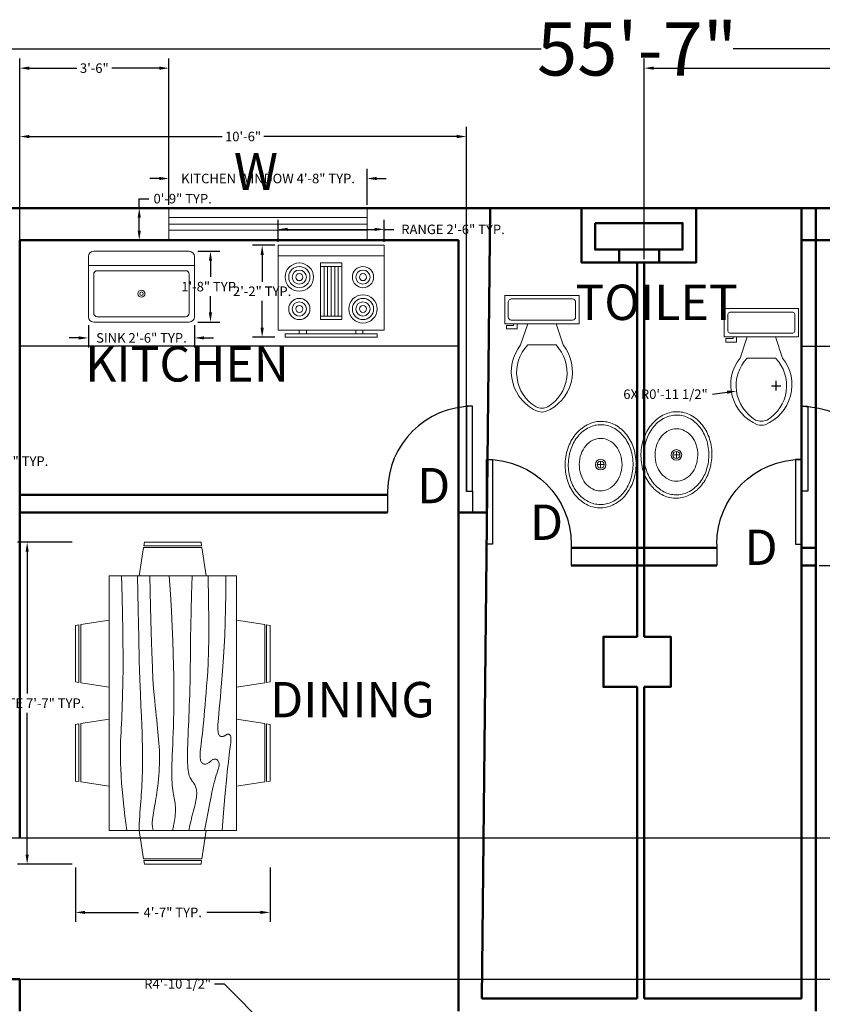
# Model space of a CAD drawing. Units: inches. Extents: x -15 to 796, y 111 to 651.
# Tile 4 of 6: x 189 to 416, y 373 to 651. Entities that reach past the tile are written whole.
import ezdxf

# ---------------------------------------------------------------- set-up
doc = ezdxf.new("R2010")
doc.units = ezdxf.units.IN
doc.header["$MEASUREMENT"] = 0
doc.layers.get('0').update_dxf_attribs({"color": 1})
for name, color, linetype, lineweight in [('A-ANNO-DIMS', 2, 'Continuous', 18), ('A-ANNO-TEXT', 7, 'Continuous', 18), ('A-AREA-IDEN', 7, 'Continuous', 25), ('A-COLS', 1, 'Continuous', 50), ('A-DOOR', 3, 'Continuous', 25), ('A-EQPM', 8, 'Continuous', 20), ('A-FLOR-CASE', 8, 'Continuous', 25), ('A-FLOR-FIXT', 9, 'Continuous', 20), ('A-FLOR-PATT', 18, 'Continuous', 13), ('A-FURN', 8, 'Continuous', 18), ('A-GLAZ', 4, 'Continuous', 18), ('A-WALL', 7, 'Continuous', 50)]:
    doc.layers.add(name, color=color, linetype=linetype, lineweight=lineweight)
doc.styles.get("Standard").update_dxf_attribs({"font": 'arial.ttf'})
doc.dimstyles.get("Standard").update_dxf_attribs({"dimscale": 15, "dimtxt": 0.18, "dimasz": 0.18, "dimexe": 0.18, "dimexo": 0.0625, "dimgap": 0.09, "dimtad": 0, "dimtih": 1, "dimtoh": 1, "dimdec": 0, "dimzin": 0, "dimdsep": 46, "dimlunit": 3, "dimtxsty": 'Standard', "dimcen": 0.09, "dimadec": 0, "dimazin": 0, "dimtfac": 1, "dimtdec": 0, "dimtofl": 0, "dimtmove": 0, "dimatfit": 3, "dimfxl": 1, "dimtolj": 1, "dimtzin": 0, "dimarcsym": 0})

# ---------------------------------------------------------------- blocks, each defined once
blk = doc.blocks.new('*U4')
for p, q in [((0, 0), (0, -6)), ((-40, 0), (-40, -6))]:
    blk.add_line(p, q)
blk.add_lwpolyline([(0, 0), (0, 40), (-1.75, 40), (-1.75, 0)], close=True)
blk.add_arc((0, 0), 40, 90, 180)
blk = doc.blocks.new('Range-Oven - 30 in top')
for p, q in [((0, -3), (30, -3)), ((12, -6), (18, -6)), ((13, -20), (13, -6)), ((14, -6), (14, -20)), ((15, -20), (15, -6)), ((16, -6), (16, -20)), ((17, -20), (17, -6)), ((18, -20), (12, -20)), ((6, -24), (6, -25)), ((8, -25), (8, -24)), ((22, -25), (22, -24)), ((24, -24), (24, -25))]:
    blk.add_line(p, q)
for points in [[(0, -24), (0, 0), (30, 0), (30, -24)], [(12, -21), (12, -5), (18, -5), (18, -21)], [(2, -26), (2, -25), (28, -25), (28, -26)]]:
    blk.add_lwpolyline(points, close=True)
for centre, radius in [((6, -9), 4), ((6, -9), 3), ((6, -9), 2), ((6, -9), 1), ((24, -9), 3), ((24, -9), 2), ((24, -9), 1), ((6, -18), 3), ((6, -18), 2), ((24, -18), 4), ((24, -18), 3), ((24, -18), 2), ((6, -18), 1), ((24, -18), 1)]:
    blk.add_circle(centre, radius)
blk = doc.blocks.new('Sink-single - 30 in top')
blk.add_line((-15, -3.999996), (15, -3.999996))
for points in [[(-13.5, 0), (13.5, 0)], [(-15, -18.499996), (-15, -1.5)], [(15, -1.5), (15, -18.499996)], [(-12.5, -5.499996), (12.5, -5.499996)], [(-13.5, -17.499996), (-13.5, -6.499996)], [(13.5, -6.499996), (13.5, -17.499996)], [(12.5, -18.499996), (-12.5, -18.499996)], [(13.5, -19.999996), (-13.5, -19.999996)]]:
    blk.add_lwpolyline(points)
for radius in [1, 0.5]:
    blk.add_circle((0, -11.999996), radius)
for centre, radius, start, end in [((-13.5, -1.5), 1.5, 90, 180), ((13.5, -1.5), 1.5, 0, 90), ((-12.5, -6.499996), 1, 90, 180), ((12.5, -6.499996), 1, 0, 90), ((-13.5, -18.499996), 1.5, 180, 270), ((-12.5, -17.499996), 1, 180, 270), ((12.5, -17.499996), 1, 270, 0), ((13.5, -18.499996), 1.5, 270, 0)]:
    blk.add_arc(centre, radius, start, end)
blk = doc.blocks.new('*U13')
for p, q in [((-24, 0), (-24, -6)), ((0, 0), (0, -6))]:
    blk.add_line(p, q)
blk.add_lwpolyline([(0, 0), (0, 24), (-1.75, 24), (-1.75, 0)], close=True)
blk.add_arc((0, 0), 24, 90, 180)
blk = doc.blocks.new('Dining Set - 36 x 72 in.')
for p, q in [((-22.2343, 26.00059), (-23.4847, 17.99762)), ((-22.2304, 26), (-5.7608, 26)), ((-22, 27.5), (-22.1562, 26.50042)), ((-5.8416, 26.5), (-22.1534, 26.5)), ((-22, 27.5), (-6, 27.5)), ((-5.8437, 26.49966), (-6, 27.5)), ((-4.5152, 17.99762), (-5.7655, 25.99926)), ((5.7657, 26.00059), (4.5153, 17.99762)), ((5.7696, 26), (22.2392, 26)), ((6, 27.5), (5.8438, 26.50042)), ((22.1584, 26.5), (5.8466, 26.5)), ((6, 27.5), (22, 27.5)), ((22.1563, 26.49966), (22, 27.5)), ((23.4848, 17.99762), (22.2345, 25.99926)), ((36, 18), (-36, 18)), ((-36, 18), (-36, -18)), ((36, -18), (36, 18)), ((-44.0006, 8.23428), (-35.9976, 9.48474)), ((44.0006, 8.23428), (35.9976, 9.48474)), ((-45.5, 8), (-44.5004, 8.15617)), ((-45.5, 8), (-45.5, -8)), ((-44.5, -8.15843), (-44.5, 8.15338)), ((-44, 8.23041), (-44, -8.23915)), ((44, 8.23041), (44, -8.23915)), ((44.5, -8.15843), (44.5, 8.15338)), ((45.5, 8), (44.5005, 8.15617)), ((45.5, 8), (45.5, -8)), ((-44.4997, -8.15631), (-45.5, -8)), ((-35.9976, -9.48476), (-43.9993, -8.2345)), ((35.9976, -9.48476), (43.9993, -8.2345)), ((44.4997, -8.15631), (45.5, -8)), ((-36, -18), (36, -18)), ((-22.2343, -26.0006), (-23.4847, -17.99762)), ((-4.5152, -17.99762), (-5.7655, -25.99928)), ((5.7657, -26.0006), (4.5153, -17.99762)), ((23.4848, -17.99762), (22.2345, -25.99928)), ((-22.2304, -26), (-5.7608, -26)), ((-22, -27.5), (-22.1562, -26.50044)), ((-5.8416, -26.5), (-22.1534, -26.5)), ((-22, -27.5), (-6, -27.5)), ((-5.8437, -26.49967), (-6, -27.5)), ((5.7696, -26), (22.2392, -26)), ((6, -27.5), (5.8438, -26.50044)), ((22.1584, -26.5), (5.8466, -26.5)), ((6, -27.5), (22, -27.5)), ((22.1563, -26.49967), (22, -27.5))]:
    blk.add_line(p, q)
for points in [[(-36, 15), (-31.1772, 14.97754), (-26.8079, 14.91406), (-22.8538, 14.81543), (-19.276, 14.6875), (-16.0362, 14.53613), (-13.0957, 14.36718), (-10.4159, 14.18652), (-7.9583, 14), (-5.6904, 13.81315), (-3.6035, 13.63021), (-1.6954, 13.45508), (0.0365, 13.29166), (1.5945, 13.14388), (2.9811, 13.01562), (4.1988, 12.9108), (5.25, 12.83333), (6.1393, 12.78613), (6.8802, 12.76823), (7.4883, 12.77767), (7.9792, 12.8125), (8.3685, 12.87077), (8.6719, 12.95052), (8.9049, 13.0498), (9.0833, 13.16666), (9.2205, 13.29899), (9.3216, 13.44401), (9.3895, 13.59879), (9.4271, 13.76041), (9.4373, 13.92594), (9.4232, 14.09245), (9.3875, 14.257), (9.3333, 14.41666), (9.2638, 14.56917), (9.1836, 14.71484), (9.0975, 14.85465), (9.0104, 14.98958), (8.9272, 15.1206), (8.8529, 15.2487), (8.7922, 15.37483), (8.75, 15.5), (8.7305, 15.62467), (8.7344, 15.74739), (8.7617, 15.86621), (8.8125, 15.97916), (8.8867, 16.08431), (8.9844, 16.17968), (9.1055, 16.26334), (9.25, 16.33333), (9.4189, 16.38802), (9.6172, 16.42708), (9.8506, 16.45052), (10.125, 16.45833), (10.4463, 16.45052), (10.8203, 16.42708), (11.2529, 16.38802), (11.75, 16.33333), (12.3184, 16.26318), (12.9694, 16.17838), (13.7151, 16.07991), (14.5677, 15.96875), (15.5395, 15.84586), (16.6426, 15.71224), (17.8893, 15.56884), (19.2917, 15.41666), (20.859, 15.25667), (22.5879, 15.08984), (24.4721, 14.91715), (26.5052, 14.73958), (28.6809, 14.5581), (30.9929, 14.3737), (33.4347, 14.18733), (36, 14)], [(-36, 10), (-28.9766, 10.14274), (-23.1725, 10.20442), (-18.4241, 10.19775), (-14.5677, 10.13541), (-11.4399, 10.03011), (-8.877, 9.89453), (-6.7154, 9.74137), (-4.7917, 9.58333), (-2.9698, 9.43082), (-1.2246, 9.28515), (0.4415, 9.14534), (2.026, 9.01041), (3.5266, 8.87939), (4.9408, 8.7513), (6.266, 8.62516), (7.5, 8.5), (8.6411, 8.37549), (9.6914, 8.2539), (10.6538, 8.13818), (11.5312, 8.03125), (12.3267, 7.93603), (13.043, 7.85547), (13.6831, 7.79248), (14.25, 7.75), (14.7471, 7.7303), (15.1797, 7.73307), (15.5537, 7.75732), (15.875, 7.80208), (16.1494, 7.86637), (16.3828, 7.94922), (16.5811, 8.04964), (16.75, 8.16666), (16.8944, 8.29915), (17.0143, 8.44531), (17.1089, 8.60319), (17.1771, 8.77083), (17.218, 8.94629), (17.2305, 9.1276), (17.2137, 9.31282), (17.1667, 9.5), (17.0895, 9.6875), (16.987, 9.875), (16.8649, 10.0625), (16.7292, 10.25), (16.5856, 10.4375), (16.4401, 10.625), (16.2985, 10.8125), (16.1667, 11), (16.05, 11.18733), (15.9518, 11.3737), (15.8752, 11.5581), (15.8229, 11.73958), (15.798, 11.91715), (15.8034, 12.08984), (15.842, 12.25667), (15.9167, 12.41666), (16.0295, 12.56836), (16.1784, 12.70833), (16.3605, 12.83268), (16.5729, 12.9375), (16.8127, 13.01888), (17.0768, 13.07291), (17.3625, 13.0957), (17.6667, 13.08333), (17.9894, 13.03312), (18.3418, 12.94726), (18.7382, 12.82918), (19.1927, 12.68229), (19.7195, 12.51001), (20.3327, 12.31575), (21.0465, 12.10294), (21.875, 11.875), (22.8357, 11.63354), (23.959, 11.37304), (25.2786, 11.08618), (26.8282, 10.76562), (28.6414, 10.40405), (30.752, 9.99414), (33.1936, 9.52856), (36, 9)], [(-36, 5.5), (-30.7157, 5.3348), (-26.069, 5.20963), (-21.9946, 5.11767), (-18.4271, 5.05208), (-15.3009, 5.00602), (-12.5508, 4.97265), (-10.1112, 4.94515), (-7.9167, 4.91666), (-5.909, 4.88167), (-4.0586, 4.83984), (-2.3429, 4.79215), (-0.7396, 4.73958), (0.7739, 4.6831), (2.22, 4.6237), (3.6213, 4.56233), (5, 4.5), (6.373, 4.43782), (7.7344, 4.3776), (9.0723, 4.32129), (10.375, 4.27083), (11.6309, 4.22819), (12.8281, 4.19531), (13.9551, 4.17415), (15, 4.16666), (15.954, 4.17448), (16.819, 4.19791), (17.6001, 4.23698), (18.3021, 4.29166), (18.9299, 4.36198), (19.4883, 4.44791), (19.9823, 4.54948), (20.4167, 4.66666), (20.7969, 4.79899), (21.1302, 4.94401), (21.4245, 5.09879), (21.6875, 5.26041), (21.9271, 5.42594), (22.1511, 5.59245), (22.3672, 5.757), (22.5834, 5.91666), (22.8065, 6.06868), (23.0404, 6.21093), (23.2879, 6.34147), (23.5521, 6.45833), (23.8358, 6.55957), (24.142, 6.64323), (24.4735, 6.70735), (24.8334, 6.75), (25.2235, 6.76969), (25.642, 6.76692), (26.0858, 6.74267), (26.5521, 6.69791), (27.0379, 6.63362), (27.5404, 6.55078), (28.0565, 6.45036), (28.5834, 6.33333), (29.1242, 6.19987), (29.7071, 6.04687), (30.3661, 5.87044), (31.1354, 5.66666), (32.0493, 5.43164), (33.142, 5.16146), (34.4475, 4.85221), (36, 4.5)], [(-36, -1), (-30.7915, -0.6591), (-26.0195, -0.38216), (-21.6519, -0.16284), (-17.6563, 0.00521), (-14.0005, 0.12833), (-10.6523, 0.21289), (-7.5796, 0.26522), (-4.75, 0.29166), (-2.134, 0.29793), (0.2878, 0.28711), (2.5317, 0.26163), (4.6146, 0.22396), (6.5529, 0.17651), (8.3633, 0.12174), (10.0623, 0.06209), (11.6667, 0), (13.1899, -0.06201), (14.6341, -0.1211), (15.9982, -0.17432), (17.2813, -0.21875), (18.4823, -0.25147), (19.6003, -0.26953), (20.6343, -0.27002), (21.5834, -0.25), (22.4481, -0.20768), (23.2357, -0.14584), (23.9549, -0.06836), (24.6146, 0.02083), (25.2235, 0.11784), (25.7904, 0.21875), (26.3241, 0.31966), (26.8334, 0.41666), (27.3265, 0.50618), (27.8099, 0.58593), (28.2894, 0.65397), (28.7709, 0.70833), (29.2601, 0.74707), (29.763, 0.76823), (30.2855, 0.76985), (30.8334, 0.75), (31.4088, 0.70784), (31.9994, 0.64713), (32.589, 0.57275), (33.1615, 0.48958), (33.7008, 0.4025), (34.1908, 0.3164), (34.6153, 0.23616), (34.9584, 0.16666), (35.2099, 0.11165), (35.3848, 0.07031), (35.504, 0.04069), (35.5886, 0.02083), (35.6594, 0.00879), (35.7377, 0.0026), (35.8442, 0.00032), (36, 0)], [(-36, -6.5), (-27.1843, -6.31267), (-20.084, -6.1263), (-14.469, -5.9419), (-10.1094, -5.76042), (-6.7752, -5.58285), (-4.2363, -5.41016), (-2.2629, -5.24333), (-0.625, -5.08334), (0.8708, -4.93099), (2.2715, -4.78646), (3.5872, -4.64974), (4.8281, -4.52084), (6.0046, -4.39974), (7.127, -4.28646), (8.2053, -4.18099), (9.25, -4.08334), (10.2705, -3.99382), (11.2734, -3.91407), (12.2647, -3.84603), (13.25, -3.79167), (14.2354, -3.75293), (15.2266, -3.73177), (16.2295, -3.73015), (17.25, -3.75), (18.2912, -3.79248), (19.3451, -3.85547), (20.4009, -3.93604), (21.4479, -4.03125), (22.4754, -4.13819), (23.4727, -4.25391), (24.4289, -4.37549), (25.3334, -4.5), (26.1785, -4.62492), (26.9694, -4.74935), (27.7145, -4.87281), (28.4219, -4.99479), (29.1, -5.11483), (29.7572, -5.23242), (30.4016, -5.34709), (31.0417, -5.45834), (31.6837, -5.56437), (32.3262, -5.65821), (32.9658, -5.73153), (33.599, -5.77604), (34.2224, -5.78345), (34.8327, -5.74545), (35.4264, -5.65373), (36, -5.5)], [(-36, -10), (-26.4022, -9.81299), (-18.4675, -9.62891), (-11.9839, -9.45069), (-6.7396, -9.28125), (-2.5226, -9.12354), (0.8789, -8.98047), (3.6769, -8.85498), (6.0833, -8.75), (8.2767, -8.66765), (10.3021, -8.60677), (12.1712, -8.56543), (13.8958, -8.54167), (15.4876, -8.53353), (16.9583, -8.53907), (18.3197, -8.55632), (19.5834, -8.58334), (20.7616, -8.61841), (21.8685, -8.66081), (22.9188, -8.71004), (23.9271, -8.76563), (24.9081, -8.82707), (25.8763, -8.89388), (26.8465, -8.96558), (27.8334, -9.04167), (28.8474, -9.12118), (29.8828, -9.20117), (30.93, -9.27824), (31.9792, -9.34896), (33.0205, -9.40991), (34.0443, -9.45768), (35.0407, -9.48885), (36, -9.5)], [(-36, -14.5), (-30.0881, -14.33513), (-25.0332, -14.21224), (-20.7312, -14.12647), (-17.0781, -14.07292), (-13.97, -14.04671), (-11.3027, -14.04297), (-8.9724, -14.05681), (-6.875, -14.08334), (-4.9224, -14.11833), (-3.0905, -14.16016), (-1.3709, -14.20785), (0.2448, -14.26042), (1.7647, -14.3169), (3.1973, -14.3763), (4.5507, -14.43767), (5.8333, -14.5), (7.0554, -14.5621), (8.235, -14.62175), (9.3922, -14.67652), (10.5469, -14.72396), (11.7192, -14.76164), (12.929, -14.78711), (14.1965, -14.79794), (15.5417, -14.79167), (16.9933, -14.76424), (18.6152, -14.70508), (20.4804, -14.60197), (22.6615, -14.44271), (25.2312, -14.21509), (28.2624, -13.9069), (31.8277, -13.50594), (36, -13)]]:
    blk.add_lwpolyline(points)
blk = doc.blocks.new('Sink - Oval top')
for p, q in [((-1, 0), (1, 0)), ((0, 1), (0, -1))]:
    blk.add_line(p, q)
for points in [[(-12.23, 0.39, 0.117634), (-11.46, -3.36, 0.104469), (-8.88, -6.8, 0.090016), (-5.08, -9.07, 0.08192), (-0.32, -10.02, 0.08192), (4.49, -9.38, 0.090016), (8.42, -7.36, 0.104469), (11.22, -4.09, 0.117634), (12.23, -0.39, 0.117634), (11.46, 3.36, 0.104469), (8.88, 6.8, 0.090016), (5.08, 9.07, 0.08192), (0.32, 10.02, 0.08192), (-4.49, 9.38, 0.090016), (-8.42, 7.36, 0.104469), (-11.22, 4.09, 0.117634)], [(-11.29, 0.16, 0.118622), (-10.52, -3.25, 0.104678), (-8.07, -6.36, 0.089562), (-4.54, -8.37, 0.081185), (-0.13, -9.15, 0.081185), (4.3, -8.49, 0.089562), (7.89, -6.58, 0.104678), (10.42, -3.55, 0.118622), (11.29, -0.16, 0.118622), (10.52, 3.25, 0.104678), (8.07, 6.36, 0.089562), (4.54, 8.37, 0.081185), (0.13, 9.15, 0.081185), (-4.3, 8.49, 0.089562), (-7.89, 6.58, 0.104678), (-10.42, 3.55, 0.118622)], [(-7.42, 0.08, 0.118283), (-6.91, -2.17, 0.104607), (-5.29, -4.21, 0.089718), (-2.97, -5.53, 0.081436), (-0.07, -6.04, 0.081436), (2.84, -5.59, 0.089718), (5.2, -4.33, 0.104607), (6.86, -2.32, 0.118283), (7.42, -0.08, 0.118283), (6.91, 2.17, 0.104607), (5.29, 4.21, 0.089718), (2.97, 5.53, 0.081436), (0.07, 6.04, 0.081436), (-2.84, 5.59, 0.089718), (-5.2, 4.33, 0.104607), (-6.86, 2.32, 0.118283)]]:
    blk.add_lwpolyline(points, format="xyb", close=True)
for radius in [1.5, 1]:
    blk.add_circle((0, 0), radius)
blk = doc.blocks.new('Toilet - top')
for p, q in [((9.5, -6), (9.5, -2)), ((-8, -8.5), (-8, -8)), ((-7, -8), (-7, -9.5)), ((-4, -8), (-6, -14)), ((4, -8), (6, -14)), ((-10, -8.5), (-8, -8.5)), ((-10, -9.5), (-10, -8.5)), ((-7, -9.5), (-10, -9.5)), ((4, -14), (-4, -14))]:
    blk.add_line(p, q)
blk.add_lwpolyline([(10.5, -8), (10.5, 0), (-10.5, 0), (-10.5, -8)], close=True)
for points in [[(-9.5, -2), (-9.5, -6)], [(8.5, -1), (-8.5, -1)], [(-8.5, -7), (8.5, -7)]]:
    blk.add_lwpolyline(points)
for centre, radius, start, end in [((-8.62, -1.88), 0.884, 81.8699, 188.1301), ((8.62, -1.88), 0.884, 351.8699, 98.1301), ((-8.62, -6.12), 0.884, 171.8699, 278.1301), ((8.62, -6.12), 0.884, 261.8699, 8.1301), ((3.52, -21.58), 12.17, 141.4691, 247.9714), ((4.2, -21.82), 11.33, 136.3677, 238.9468), ((-3.52, -21.58), 12.17, 292.0284, 38.5307), ((-4.2, -21.82), 11.33, 301.053, 43.6321), ((0, -27.88), 4, 245.7318, 294.2682), ((0, -29), 4, 254.8605, 285.1395)]:
    blk.add_arc(centre, radius, start, end)
blk = doc.blocks.new('*U15')
for p, q in [((0, 0), (0, -6)), ((24, 0), (24, -6))]:
    blk.add_line(p, q)
blk.add_lwpolyline([(0, 0), (0, 24), (1.75, 24), (1.75, 0)], close=True)
blk.add_arc((0, 0), 24, 0, 90)
blk = doc.blocks.new('*D16')
at = {"layer": 'A-ANNO-DIMS', "color": 0, "lineweight": -2, "transparency": 16777216}
for p, q in [((30.18, 599.06), (30.18, 645.85)), ((697.18, 599.06), (697.18, 645.85)), ((32.88, 643.15), (336.57, 643.15)), ((694.48, 643.15), (390.8, 643.15))]:
    blk.add_line(p, q, dxfattribs=at)
at = {"layer": 'A-ANNO-DIMS', "color": 0, "transparency": 16777216}
for points in [[(32.88, 643.6), (32.88, 642.7), (30.18, 643.15)], [(694.48, 643.6), (694.48, 642.7), (697.18, 643.15)]]:
    blk.add_solid(points, dxfattribs=at)
at = {"layer": 'Defpoints', "color": 0, "transparency": 16777216}
for p in [(697.18, 643.15), (30.18, 598.13), (697.18, 598.13)]:
    blk.add_point(p, dxfattribs=at)
at = {"layer": 'A-ANNO-DIMS', "color": 0, "transparency": 16777216, "insert": (363.68, 643.15), "char_height": 2.7, "attachment_point": 5}
blk.add_mtext('\\A1;{\\H5.55556x;55\'-7"}', dxfattribs=at)
blk = doc.blocks.new('*D22')
at = {"layer": 'A-ANNO-DIMS', "color": 0, "lineweight": -2, "transparency": 16777216}
for p, q in [((189.18, 518.06), (189.18, 621.1)), ((315.43, 518.06), (315.43, 621.1)), ((191.88, 618.4), (246.45, 618.4)), ((312.73, 618.4), (258.17, 618.4))]:
    blk.add_line(p, q, dxfattribs=at)
at = {"layer": 'A-ANNO-DIMS', "color": 0, "transparency": 16777216}
for points in [[(191.88, 618.85), (191.88, 617.95), (189.18, 618.4)], [(312.73, 618.85), (312.73, 617.95), (315.43, 618.4)]]:
    blk.add_solid(points, dxfattribs=at)
at = {"layer": 'Defpoints', "color": 0, "transparency": 16777216}
for p in [(315.43, 618.4), (189.18, 517.13), (315.43, 517.13)]:
    blk.add_point(p, dxfattribs=at)
at = {"layer": 'A-ANNO-DIMS', "color": 0, "transparency": 16777216, "insert": (252.31, 618.4), "char_height": 2.7, "attachment_point": 5}
blk.add_mtext('\\A1;10\'-6"', dxfattribs=at)
blk = doc.blocks.new('WIN-KITCHEN-56IN')
for p, q in [((0, 6.34), (56, 6.34)), ((0, 4.5), (56, 4.5)), ((0, 2.84), (56, 2.84))]:
    blk.add_line(p, q)
blk.add_lwpolyline([(0, 9), (56, 9), (56, 0), (0, 0)], close=True)
blk = doc.blocks.new('*D45')
at = {"layer": 'A-ANNO-DIMS', "color": 0, "lineweight": -2, "transparency": 16777216}
for p, q in [((134.03, 529.37), (134.03, 523.92)), ((158.58, 529.37), (158.58, 523.92)), ((136.73, 526.62), (155.88, 526.62)), ((158.58, 526.62), (161.28, 526.62))]:
    blk.add_line(p, q, dxfattribs=at)
at = {"layer": 'A-ANNO-DIMS', "color": 0, "transparency": 16777216}
for points in [[(136.73, 527.07), (136.73, 526.17), (134.03, 526.62)], [(155.88, 527.07), (155.88, 526.17), (158.58, 526.62)]]:
    blk.add_solid(points, dxfattribs=at)
at = {"layer": 'Defpoints', "color": 0, "transparency": 16777216}
for p in [(134.03, 530.3), (158.58, 530.3), (158.58, 526.62)]:
    blk.add_point(p, dxfattribs=at)
at = {"layer": 'A-ANNO-DIMS', "color": 0, "transparency": 16777216, "insert": (180.13, 526.62), "char_height": 2.7, "attachment_point": 5}
blk.add_mtext('\\A1;BASIN 2\'-0 1/2" TYP.', dxfattribs=at)
blk = doc.blocks.new('*D51')
at = {"layer": 'A-ANNO-DIMS', "color": 0, "lineweight": -2, "transparency": 16777216}
for p, q in [((262.21, 588.59), (262.21, 594.85)), ((292.21, 588.59), (292.21, 594.85)), ((264.91, 592.15), (289.51, 592.15)), ((292.21, 592.15), (294.91, 592.15))]:
    blk.add_line(p, q, dxfattribs=at)
at = {"layer": 'A-ANNO-DIMS', "color": 0, "transparency": 16777216}
for points in [[(264.91, 592.6), (264.91, 591.7), (262.21, 592.15)], [(289.51, 592.6), (289.51, 591.7), (292.21, 592.15)]]:
    blk.add_solid(points, dxfattribs=at)
at = {"layer": 'Defpoints', "color": 0, "transparency": 16777216}
for p in [(292.21, 592.15), (262.21, 587.65), (292.21, 587.65)]:
    blk.add_point(p, dxfattribs=at)
at = {"layer": 'A-ANNO-DIMS', "color": 0, "transparency": 16777216, "insert": (311.65, 592.15), "char_height": 2.7, "attachment_point": 5}
blk.add_mtext('\\A1;RANGE 2\'-6" TYP.', dxfattribs=at)
blk = doc.blocks.new('*D52')
at = {"layer": 'A-ANNO-DIMS', "color": 0, "lineweight": -2, "transparency": 16777216}
for p, q in [((261.28, 587.65), (255.01, 587.65)), ((257.71, 584.95), (257.71, 577.36)), ((257.71, 564.35), (257.71, 571.94)), ((261.28, 561.65), (255.01, 561.65))]:
    blk.add_line(p, q, dxfattribs=at)
at = {"layer": 'A-ANNO-DIMS', "color": 0, "transparency": 16777216}
for points in [[(257.26, 584.95), (258.16, 584.95), (257.71, 587.65)], [(257.26, 564.35), (258.16, 564.35), (257.71, 561.65)]]:
    blk.add_solid(points, dxfattribs=at)
at = {"layer": 'Defpoints', "color": 0, "transparency": 16777216}
for p in [(257.71, 587.65), (262.21, 587.65), (262.21, 561.65)]:
    blk.add_point(p, dxfattribs=at)
at = {"layer": 'A-ANNO-DIMS', "color": 0, "transparency": 16777216, "insert": (257.71, 574.65), "char_height": 2.7, "attachment_point": 5}
blk.add_mtext('\\A1;2\'-2" TYP.', dxfattribs=at)
blk = doc.blocks.new('*D53')
at = {"layer": 'A-ANNO-DIMS', "color": 0, "lineweight": -2, "transparency": 16777216}
for p, q in [((208.59, 565.02), (208.59, 558.76)), ((238.59, 565.02), (238.59, 558.76)), ((205.89, 561.46), (203.19, 561.46)), ((241.29, 561.46), (243.99, 561.46))]:
    blk.add_line(p, q, dxfattribs=at)
at = {"layer": 'A-ANNO-DIMS', "color": 0, "transparency": 16777216}
for points in [[(205.89, 561.91), (205.89, 561.01), (208.59, 561.46)], [(241.29, 561.91), (241.29, 561.01), (238.59, 561.46)]]:
    blk.add_solid(points, dxfattribs=at)
at = {"layer": 'Defpoints', "color": 0, "transparency": 16777216}
for p in [(208.59, 565.96), (238.59, 565.96), (238.59, 561.46)]:
    blk.add_point(p, dxfattribs=at)
at = {"layer": 'A-ANNO-DIMS', "color": 0, "transparency": 16777216, "insert": (223.59, 561.46), "char_height": 2.7, "attachment_point": 5}
blk.add_mtext('\\A1;SINK 2\'-6" TYP.', dxfattribs=at)
blk = doc.blocks.new('*D54')
at = {"layer": 'A-ANNO-DIMS', "color": 0, "lineweight": -2, "transparency": 16777216}
for p, q in [((239.53, 585.96), (245.79, 585.96)), ((243.09, 583.26), (243.09, 578.69)), ((243.09, 568.66), (243.09, 573.23)), ((239.53, 565.96), (245.79, 565.96))]:
    blk.add_line(p, q, dxfattribs=at)
at = {"layer": 'A-ANNO-DIMS', "color": 0, "transparency": 16777216}
for points in [[(242.64, 583.26), (243.54, 583.26), (243.09, 585.96)], [(242.64, 568.66), (243.54, 568.66), (243.09, 565.96)]]:
    blk.add_solid(points, dxfattribs=at)
at = {"layer": 'Defpoints', "color": 0, "transparency": 16777216}
for p in [(238.59, 585.96), (243.09, 585.96), (238.59, 565.96)]:
    blk.add_point(p, dxfattribs=at)
at = {"layer": 'A-ANNO-DIMS', "color": 0, "transparency": 16777216, "insert": (243.09, 575.96), "char_height": 2.7, "attachment_point": 5}
blk.add_mtext('\\A1;1\'-8" TYP.', dxfattribs=at)
blk = doc.blocks.new('*D55')
at = {"layer": 'A-ANNO-DIMS', "color": 0, "lineweight": -2, "transparency": 16777216}
for p, q in [((204, 503.69), (188.59, 503.69)), ((191.29, 500.99), (191.29, 460.89)), ((191.29, 415.39), (191.29, 455.48)), ((204, 412.69), (188.59, 412.69))]:
    blk.add_line(p, q, dxfattribs=at)
at = {"layer": 'A-ANNO-DIMS', "color": 0, "transparency": 16777216}
for points in [[(190.84, 500.99), (191.74, 500.99), (191.29, 503.69)], [(190.84, 415.39), (191.74, 415.39), (191.29, 412.69)]]:
    blk.add_solid(points, dxfattribs=at)
at = {"layer": 'Defpoints', "color": 0, "transparency": 16777216}
for p in [(204.94, 503.69), (191.29, 412.69), (204.94, 412.69)]:
    blk.add_point(p, dxfattribs=at)
at = {"layer": 'A-ANNO-DIMS', "color": 0, "transparency": 16777216, "insert": (191.29, 458.19), "char_height": 2.7, "attachment_point": 5}
blk.add_mtext('\\A1;DINETTE 7\'-7" TYP.', dxfattribs=at)
blk = doc.blocks.new('*D56')
at = {"layer": 'A-ANNO-DIMS', "color": 0, "lineweight": -2, "transparency": 16777216}
for p, q in [((204.94, 411.75), (204.94, 396.34)), ((259.94, 411.75), (259.94, 396.34)), ((207.64, 399.04), (222.8, 399.04)), ((257.24, 399.04), (242.07, 399.04))]:
    blk.add_line(p, q, dxfattribs=at)
at = {"layer": 'A-ANNO-DIMS', "color": 0, "transparency": 16777216}
for points in [[(207.64, 399.49), (207.64, 398.59), (204.94, 399.04)], [(257.24, 399.49), (257.24, 398.59), (259.94, 399.04)]]:
    blk.add_solid(points, dxfattribs=at)
at = {"layer": 'Defpoints', "color": 0, "transparency": 16777216}
for p in [(204.94, 412.69), (259.94, 412.69), (259.94, 399.04)]:
    blk.add_point(p, dxfattribs=at)
at = {"layer": 'A-ANNO-DIMS', "color": 0, "transparency": 16777216, "insert": (232.44, 399.04), "char_height": 2.7, "attachment_point": 5}
blk.add_mtext('\\A1;4\'-7" TYP.', dxfattribs=at)
blk = doc.blocks.new('*D61')
at = {"layer": 'A-ANNO-DIMS', "color": 0, "lineweight": -2, "transparency": 16777216}
for p, q in [((231.37, 599.06), (231.37, 609.23)), ((287.37, 599.06), (287.37, 609.23)), ((228.67, 606.53), (225.97, 606.53)), ((290.07, 606.53), (292.77, 606.53))]:
    blk.add_line(p, q, dxfattribs=at)
at = {"layer": 'A-ANNO-DIMS', "color": 0, "transparency": 16777216}
for points in [[(228.67, 606.98), (228.67, 606.08), (231.37, 606.53)], [(290.07, 606.98), (290.07, 606.08), (287.37, 606.53)]]:
    blk.add_solid(points, dxfattribs=at)
at = {"layer": 'Defpoints', "color": 0, "transparency": 16777216}
for p in [(287.37, 606.53), (231.37, 598.13), (287.37, 598.13)]:
    blk.add_point(p, dxfattribs=at)
at = {"layer": 'A-ANNO-DIMS', "color": 0, "transparency": 16777216, "insert": (259.37, 606.53), "char_height": 2.7, "attachment_point": 5}
blk.add_mtext('\\A1;KITCHEN WINDOW 4\'-8" TYP.', dxfattribs=at)
blk = doc.blocks.new('*D62')
at = {"layer": 'A-ANNO-DIMS', "color": 0, "lineweight": -2, "transparency": 16777216}
for p, q in [((222.97, 598.13), (222.97, 600.83)), ((222.97, 600.83), (225.67, 600.83)), ((230.43, 598.13), (220.27, 598.13)), ((222.97, 591.83), (222.97, 595.43)), ((230.43, 589.13), (220.27, 589.13))]:
    blk.add_line(p, q, dxfattribs=at)
at = {"layer": 'A-ANNO-DIMS', "color": 0, "transparency": 16777216}
for points in [[(222.52, 595.43), (223.42, 595.43), (222.97, 598.13)], [(222.52, 591.83), (223.42, 591.83), (222.97, 589.13)]]:
    blk.add_solid(points, dxfattribs=at)
at = {"layer": 'Defpoints', "color": 0, "transparency": 16777216}
for p in [(222.97, 598.13), (231.37, 598.13), (231.37, 589.13)]:
    blk.add_point(p, dxfattribs=at)
at = {"layer": 'A-ANNO-DIMS', "color": 0, "transparency": 16777216, "insert": (235.24, 600.83), "char_height": 2.7, "attachment_point": 5}
blk.add_mtext('\\A1;0\'-9" TYP.', dxfattribs=at)
blk = doc.blocks.new('*D75')
at = {"layer": 'A-ANNO-DIMS', "color": 0, "lineweight": -2, "transparency": 16777216}
for p, q in [((415.12, 598.13), (739.48, 598.13)), ((736.78, 595.43), (736.78, 550.36)), ((736.78, 499.83), (736.78, 544.9)), ((415.12, 497.13), (739.48, 497.13))]:
    blk.add_line(p, q, dxfattribs=at)
at = {"layer": 'A-ANNO-DIMS', "color": 0, "transparency": 16777216}
for points in [[(736.33, 595.43), (737.23, 595.43), (736.78, 598.13)], [(736.33, 499.83), (737.23, 499.83), (736.78, 497.13)]]:
    blk.add_solid(points, dxfattribs=at)
at = {"layer": 'Defpoints', "color": 0, "transparency": 16777216}
for p in [(414.18, 598.13), (414.18, 497.13), (736.78, 497.13)]:
    blk.add_point(p, dxfattribs=at)
at = {"layer": 'A-ANNO-DIMS', "color": 0, "transparency": 16777216, "insert": (736.78, 547.63), "char_height": 2.7, "attachment_point": 5}
blk.add_mtext('\\A1;8\'-5"', dxfattribs=at)
blk = doc.blocks.new('*D76')
at = {"layer": 'A-ANNO-DIMS', "color": 0, "lineweight": -2, "transparency": 16777216}
for p, q in [((189.18, 590.06), (189.18, 640.43)), ((231.37, 599.06), (231.37, 640.43)), ((191.88, 637.73), (205.34, 637.73)), ((228.67, 637.73), (215.21, 637.73))]:
    blk.add_line(p, q, dxfattribs=at)
at = {"layer": 'A-ANNO-DIMS', "color": 0, "transparency": 16777216}
for points in [[(191.88, 638.18), (191.88, 637.28), (189.18, 637.73)], [(228.67, 638.18), (228.67, 637.28), (231.37, 637.73)]]:
    blk.add_solid(points, dxfattribs=at)
at = {"layer": 'Defpoints', "color": 0, "transparency": 16777216}
for p in [(231.37, 637.73), (231.37, 598.13), (189.18, 589.13)]:
    blk.add_point(p, dxfattribs=at)
at = {"layer": 'A-ANNO-DIMS', "color": 0, "transparency": 16777216, "insert": (210.27, 637.73), "char_height": 2.7, "attachment_point": 5}
blk.add_mtext('\\A1;3\'-6"', dxfattribs=at)
blk = doc.blocks.new('*D78')
at = {"layer": 'A-ANNO-DIMS', "color": 0, "lineweight": -2, "transparency": 16777216}
for p, q in [((185.12, 420.13), (739.48, 420.13)), ((736.78, 417.43), (736.78, 402.86)), ((736.78, 382.83), (736.78, 397.4)), ((185.87, 380.13), (739.48, 380.13))]:
    blk.add_line(p, q, dxfattribs=at)
at = {"layer": 'A-ANNO-DIMS', "color": 0, "transparency": 16777216}
for points in [[(736.33, 417.43), (737.23, 417.43), (736.78, 420.13)], [(736.33, 382.83), (737.23, 382.83), (736.78, 380.13)]]:
    blk.add_solid(points, dxfattribs=at)
at = {"layer": 'Defpoints', "color": 0, "transparency": 16777216}
for p in [(184.18, 420.13), (736.78, 420.13), (184.93, 380.13)]:
    blk.add_point(p, dxfattribs=at)
at = {"layer": 'A-ANNO-DIMS', "color": 0, "transparency": 16777216, "insert": (736.78, 400.13), "char_height": 2.7, "attachment_point": 5}
blk.add_mtext('\\A1;3\'-4"', dxfattribs=at)
blk = doc.blocks.new('*D83')
at = {"layer": 'A-ANNO-DIMS', "color": 0, "lineweight": -2, "transparency": 16777216}
for p, q in [((365.68, 583.73), (365.68, 640.43)), ((697.18, 599.06), (697.18, 640.43)), ((368.38, 637.73), (522.28, 637.73)), ((694.48, 637.73), (540.59, 637.73))]:
    blk.add_line(p, q, dxfattribs=at)
at = {"layer": 'A-ANNO-DIMS', "color": 0, "transparency": 16777216}
for points in [[(368.38, 638.18), (368.38, 637.28), (365.68, 637.73)], [(694.48, 638.18), (694.48, 637.28), (697.18, 637.73)]]:
    blk.add_solid(points, dxfattribs=at)
at = {"layer": 'Defpoints', "color": 0, "transparency": 16777216}
for p in [(697.18, 637.73), (697.18, 598.13), (365.68, 582.8)]:
    blk.add_point(p, dxfattribs=at)
at = {"layer": 'A-ANNO-DIMS', "color": 0, "transparency": 16777216, "insert": (531.43, 637.73), "char_height": 2.7, "attachment_point": 5}
blk.add_mtext('\\A1;27\'-7 1/2"', dxfattribs=at)
blk = doc.blocks.new('*D88')
at = {"layer": 'A-ANNO-DIMS', "color": 0, "lineweight": -2, "transparency": 16777216}
for p, q in [((244.25, 378.84), (246.95, 378.84)), ((246.95, 378.84), (269.95, 355.84)), ((312.02, 312.41), (314.72, 312.41)), ((313.37, 311.06), (313.37, 313.76))]:
    blk.add_line(p, q, dxfattribs=at)
at = {"layer": 'A-ANNO-DIMS', "color": 0, "transparency": 16777216}
blk.add_solid([(270.27, 356.16), (269.63, 355.52), (271.86, 353.93)], dxfattribs=at)
at = {"layer": 'Defpoints', "color": 0, "transparency": 16777216}
for p in [(271.86, 353.93), (313.37, 312.41)]:
    blk.add_point(p, dxfattribs=at)
at = {"layer": 'A-ANNO-DIMS', "color": 0, "transparency": 16777216, "insert": (233.82, 378.84), "char_height": 2.7, "attachment_point": 5}
blk.add_mtext('\\A1;R4\'-10 1/2"', dxfattribs=at)
blk = doc.blocks.new('*D90')
at = {"layer": 'A-ANNO-DIMS', "color": 0, "lineweight": -2, "transparency": 16777216}
for p, q in [((403, 546.61), (403, 549.31)), ((385.04, 545.54), (389.1, 546.09)), ((401.65, 547.96), (404.35, 547.96))]:
    blk.add_line(p, q, dxfattribs=at)
at = {"layer": 'A-ANNO-DIMS', "color": 0, "transparency": 16777216}
blk.add_solid([(389.04, 546.54), (389.16, 545.64), (391.78, 546.45)], dxfattribs=at)
at = {"layer": 'Defpoints', "color": 0, "transparency": 16777216}
for p in [(391.78, 546.45), (403, 547.96)]:
    blk.add_point(p, dxfattribs=at)
at = {"layer": 'A-ANNO-DIMS', "color": 0, "transparency": 16777216, "insert": (371.71, 545.54), "char_height": 2.7, "attachment_point": 5}
blk.add_mtext('\\A1;6X R0\'-11 1/2"', dxfattribs=at)

msp = doc.modelspace()

# ---------------------------------------------------------------- hatches: boundary and pattern name
at = {"layer": 'A-FLOR-PATT'}
h = msp.add_hatch(dxfattribs=at)
h.set_pattern_fill('_USER', color=256, scale=5, angle=90, pattern_type=0)
h.set_pattern_definition([(90, (0, 0), (-5, 3e-16), [])])
h.paths.add_polyline_path([(99.18, 589.13), (39.18, 589.13), (39.18, 529.13), (75.18, 529.13), (75.18, 530.13, -0.392996), (97.43, 554.06), (97.43, 554.13), (99.18, 554.13)])
h.paths.add_polyline_path([(688.18, 589.13), (628.18, 589.13), (628.18, 554.13), (629.93, 554.13), (629.93, 554.06, -0.392996), (652.18, 530.13), (652.18, 529.13), (688.18, 529.13)])
h.paths.add_polyline_path([(40.9, 557.57), (98.32, 557.57), (98.32, 574.06), (40.9, 574.06)], flags=24)
h.paths.add_polyline_path([(628.32, 557.57), (685.73, 557.57), (685.73, 574.06), (628.32, 574.06)], flags=24)

# ---------------------------------------------------------------- linework, layer by layer
at = {"layer": 'A-COLS'}
for points in [[(363.68, 476.96), (354.16, 476.96), (354.16, 462.8), (363.68, 462.8)], [(365.68, 462.8), (373.21, 462.8), (373.21, 476.96), (365.68, 476.96)]]:
    msp.add_lwpolyline(points, dxfattribs=at)
at = {"layer": 'A-FLOR-CASE'}
for p, q in [((313.18, 559.13), (189.18, 559.13)), ((410.18, 559.13), (538.18, 559.13))]:
    msp.add_line(p, q, dxfattribs=at)
at = {"layer": 'A-WALL'}
for p, q in [((322.48, 598.13), (30.18, 598.13)), ((322.18, 598.13), (319.78, 374.68)), ((414.18, 598.13), (322.48, 598.13)), ((405.18, 598.13), (697.18, 598.13)), ((410.18, 374.68), (410.18, 598.13)), ((414.18, 371.13), (414.18, 598.13)), ((189.18, 589.13), (189.18, 420.13)), ((313.18, 589.13), (189.18, 589.13)), ((313.18, 371.13), (313.18, 589.13)), ((410.18, 589.13), (538.18, 589.13)), ((363.68, 476.96), (363.68, 582.8)), ((365.68, 476.96), (365.68, 582.8)), ((293.18, 517.13), (189.18, 517.13)), ((293.18, 512.13), (189.18, 512.13)), ((321.26, 512.13), (313.18, 512.13)), ((386.18, 502.13), (345.09, 502.13)), ((414.18, 502.13), (410.18, 502.13)), ((386.18, 497.13), (345.09, 497.13)), ((414.18, 497.13), (410.18, 497.13)), ((363.68, 374.68), (363.68, 462.8)), ((365.68, 374.68), (365.68, 462.8)), ((189.18, 380.13), (30.18, 380.13)), ((189.18, 380.13), (189.18, 371.13)), ((313.18, 374.68), (313.18, 371.13)), ((363.68, 374.68), (319.78, 374.68)), ((410.18, 374.68), (365.68, 374.68)), ((414.18, 371.13), (414.18, 374.68))]:
    msp.add_line(p, q, dxfattribs=at)
for points in [[(347.94, 598.13), (380.4, 598.13), (380.4, 582.8), (347.94, 582.8)], [(351.82, 593.93), (376.52, 593.93), (376.52, 586.43), (351.82, 586.43)], [(358.6, 586.43), (369.96, 586.43), (369.96, 582.8), (358.6, 582.8)]]:
    msp.add_lwpolyline(points, close=True, dxfattribs=at)

# ---------------------------------------------------------------- block references
at = {"layer": 'A-DOOR'}
msp.add_blockref('*U13', (317.18, 518.13), dxfattribs=at)
at = {"layer": 'A-DOOR', "xscale": -1}
for name, p in [('*U13', (410.18, 518.13)), ('*U13', (321.09, 503.13)), ('*U15', (410.18, 503.13))]:
    msp.add_blockref(name, p, dxfattribs=at)
at = {"layer": 'A-DOOR', "xscale": -1, "rotation": 90}
msp.add_blockref('*U4', (183.18, 380.13), dxfattribs=at)
at = {"layer": 'A-EQPM'}
msp.add_blockref('Range-Oven - 30 in top', (262.21, 587.65), dxfattribs=at)
at = {"layer": 'A-FLOR-FIXT'}
for name, p in [('Sink-single - 30 in top', (223.59, 585.96)), ('Toilet - top', (336.77, 573.49)), ('Toilet - top', (398.8, 569.78))]:
    msp.add_blockref(name, p, dxfattribs=at)
for p, rotation in [((374.8, 528.37), 90), ((353.38, 525.64), 270)]:
    msp.add_blockref('Sink - Oval top', p, dxfattribs=dict(at, rotation=rotation))
at = {"layer": 'A-FURN', "rotation": 270}
msp.add_blockref('Dining Set - 36 x 72 in.', (232.44, 458.19), dxfattribs=at)
at = {"layer": 'A-GLAZ'}
msp.add_blockref('WIN-KITCHEN-56IN', (231.37, 589.13), dxfattribs=at)

# ---------------------------------------------------------------- texts
at = {"layer": 'A-ANNO-TEXT', "attachment_point": 1}
for s, width, gutter_width, insert, char_height in [('W', 19.9719, 52.27, (249.7, 613.77), 10.45), ('D', 13.2435, 1, (301.48, 524.71), 10), ('D', 13.2435, 1, (333.39, 514.35), 10), ('D', 13.2435, 1, (394.02, 507.26), 10)]:
    msp.add_mtext_dynamic_manual_height_columns(s, width=width, gutter_width=gutter_width, heights=[0], dxfattribs=dict(at, insert=insert, char_height=char_height))
at = {"layer": 'A-AREA-IDEN', "char_height": 10, "attachment_point": 1}
for s, width, insert in [('TOILET', 20.6028, (346.24, 576.52)), ('KITCHEN', 30.3121, (207.7, 559.13)), ('DINING', 31.9005, (259.94, 464.19))]:
    msp.add_mtext_dynamic_manual_height_columns(s, width=width, gutter_width=50, heights=[0], dxfattribs=dict(at, insert=insert))

# ---------------------------------------------------------------- dimensions: what is measured, and where the dimension line sits
at = {"layer": 'A-ANNO-DIMS'}
dim = msp.add_linear_dim(base=(697.18, 643.15), p1=(30.18, 598.13), p2=(697.18, 598.13), text='{\\H5.55556x;<>}', dimstyle='Standard', override={"dimclrd": 0, "dimclre": 0, "dimclrt": 0}, dxfattribs=at)
dim.commit()
dim.dimension.update_dxf_attribs({"geometry": '*D16', "text_midpoint": (363.68, 643.15), "dimtype": 160})
for base, p1, p2, override, picture, middle in [((231.37, 637.73), (189.18, 589.13), (231.37, 598.13), {"dimdec": 1, "dimlfac": 1, "dimrnd": 0, "dimzin": 1, "dimdsep": 46, "dimlunit": 4, "dimfrac": 2}, '*D76', (210.27, 637.73)), ((697.18, 637.73), (365.68, 582.8), (697.18, 598.13), {"dimdec": 1, "dimlfac": 1, "dimrnd": 0, "dimzin": 1, "dimdsep": 46, "dimlunit": 4, "dimfrac": 2}, '*D83', (531.43, 637.73)), ((315.43, 618.4), (189.18, 517.13), (315.43, 517.13), {"dimclrd": 0, "dimclre": 0, "dimclrt": 0}, '*D22', (252.31, 618.4))]:
    dim = msp.add_linear_dim(base=base, p1=p1, p2=p2, dimstyle='Standard', override=override, dxfattribs=at)
    dim.commit()
    dim.dimension.update_dxf_attribs({"geometry": picture, "text_midpoint": middle})
for base, p1, p2, text, picture, middle in [((287.37, 606.53), (231.37, 598.13), (287.37, 598.13), 'KITCHEN WINDOW <> TYP.', '*D61', (259.37, 606.53)), ((292.21, 592.15), (262.21, 587.65), (292.21, 587.65), 'RANGE <> TYP.', '*D51', (311.65, 592.15)), ((238.59, 561.46), (208.59, 565.96), (238.59, 565.96), 'SINK <> TYP.', '*D53', (223.59, 561.46)), ((158.5769, 526.6215), (134.026, 530.3042), (158.5769, 530.3042), 'BASIN <> TYP.', '*D45', (180.1253, 526.6215)), ((259.94, 399.04), (204.94, 412.69), (259.94, 412.69), '<> TYP.', '*D56', (232.44, 399.04))]:
    dim = msp.add_linear_dim(base=base, p1=p1, p2=p2, text=text, dimstyle='Standard', override={"dimdec": 1, "dimlfac": 1, "dimrnd": 0, "dimzin": 1, "dimdsep": 46, "dimlunit": 4, "dimfrac": 2}, dxfattribs=at)
    dim.commit()
    dim.dimension.update_dxf_attribs({"geometry": picture, "text_midpoint": middle})
for base, p1, p2, angle, text, picture, middle in [((222.97, 598.13), (231.37, 589.13), (231.37, 598.13), 90, '<> TYP.', '*D62', (235.24, 600.83)), ((257.71, 587.65), (262.21, 561.65), (262.21, 587.65), 90, '<> TYP.', '*D52', (257.71, 574.65)), ((243.09, 585.96), (238.59, 565.96), (238.59, 585.96), 90, '<> TYP.', '*D54', (243.09, 575.96)), ((191.29, 412.69), (204.94, 503.69), (204.94, 412.69), 270, 'DINETTE <> TYP.', '*D55', (191.29, 458.19))]:
    dim = msp.add_linear_dim(base=base, p1=p1, p2=p2, angle=angle, text=text, dimstyle='Standard', override={"dimdec": 1, "dimlfac": 1, "dimrnd": 0, "dimzin": 1, "dimdsep": 46, "dimlunit": 4, "dimfrac": 2}, dxfattribs=at)
    dim.commit()
    dim.dimension.update_dxf_attribs({"geometry": picture, "text_midpoint": middle})
for base, p1, p2, picture, middle in [((736.78, 497.13), (414.18, 598.13), (414.18, 497.13), '*D75', (736.78, 547.63)), ((736.78, 420.13), (184.93, 380.13), (184.18, 420.13), '*D78', (736.78, 400.13))]:
    dim = msp.add_linear_dim(base=base, p1=p1, p2=p2, angle=90, dimstyle='Standard', override={"dimdec": 1, "dimlfac": 1, "dimrnd": 0, "dimzin": 1, "dimdsep": 46, "dimlunit": 4, "dimfrac": 2}, dxfattribs=at)
    dim.commit()
    dim.dimension.update_dxf_attribs({"geometry": picture, "text_midpoint": middle})
dim = msp.add_radius_dim(center=(403, 547.96), mpoint=(391.78, 546.45), text='6X <>', dimstyle='Standard', override={"dimdec": 1, "dimlfac": 1, "dimrnd": 0, "dimzin": 1, "dimdsep": 46, "dimlunit": 4, "dimfrac": 2}, dxfattribs=at)
dim.commit()
dim.dimension.update_dxf_attribs({"geometry": '*D90', "text_midpoint": (385.04, 545.54), "dimtype": 164})
dim = msp.add_radius_dim(center=(313.37, 312.41), mpoint=(271.86, 353.93), dimstyle='Standard', override={"dimdec": 1, "dimlfac": 1, "dimrnd": 0, "dimzin": 1, "dimdsep": 46, "dimlunit": 4, "dimfrac": 2}, dxfattribs=at)
dim.commit()
dim.dimension.update_dxf_attribs({"geometry": '*D88', "text_midpoint": (233.82, 378.84), "dimtype": 164})

doc.saveas('drawing.dxf')
